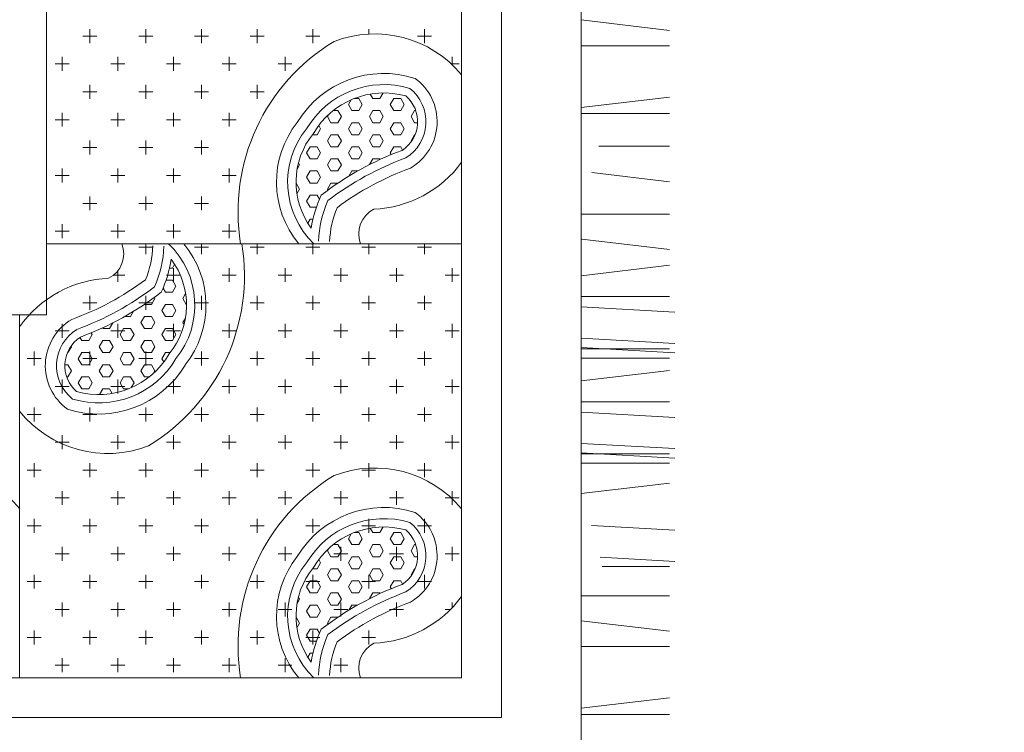
# Model space of a CAD drawing. Units: inches. Extents: x -638 to 186, y -762 to 59.
# Tile 25 of 31: x -65.6 to -46.38, y -107.92 to -94. Entities that reach past the tile are written whole.
import ezdxf

# ---------------------------------------------------------------- set-up
doc = ezdxf.new("R2010")
doc.units = ezdxf.units.IN
doc.layers.add('A-ANNO-DIMS', color=2, linetype='Continuous', lineweight=18)
doc.layers.add('furn', color=8, linetype='Continuous', lineweight=13)
doc.styles.get("Standard").update_dxf_attribs({"font": 'arial.ttf'})
doc.dimstyles.new('ISO-25', dxfattribs={"dimtxt": 4, "dimasz": 4, "dimexe": 1.25, "dimexo": 0.625, "dimtad": 0, "dimlunit": 4, "dimtxsty": 'Standard', "dimcen": 2.5, "dimclrt": 256, "dimadec": 0, "dimazin": 0, "dimtfac": 1, "dimtmove": 0, "dimatfit": 3, "dimfxl": 1, "dimfxlon": 1, "dimarcsym": 0})

# ---------------------------------------------------------------- blocks, each defined once
blk = doc.blocks.new('BED-DOUBLE-WITH-NIGHTSTANDS')
for p, q in [((58.548, 11.244), (58.548, 59.951)), ((68.982, 31.914), (68.982, 1.829)), ((67.427, 30.359), (67.427, 3.384)), ((66.65, 29.582), (66.65, 4.161)), ((68.982, 17.003), (70.71, 16.797)), ((59.394, 16.552), (59.394, 16.825)), ((60.483, 16.552), (60.483, 16.825)), ((61.571, 16.552), (61.571, 16.825)), ((62.659, 16.552), (62.659, 16.825)), ((63.748, 16.552), (63.748, 16.825)), ((64.836, 16.726), (64.836, 16.825)), ((65.924, 16.552), (65.924, 16.825)), ((59.258, 16.688), (59.53, 16.688)), ((60.346, 16.688), (60.619, 16.688)), ((61.435, 16.688), (61.707, 16.688)), ((62.523, 16.688), (62.795, 16.688)), ((63.612, 16.688), (63.884, 16.688)), ((65.788, 16.688), (66.06, 16.688)), ((68.982, 16.497), (70.707, 16.497)), ((58.85, 16.008), (58.85, 16.28)), ((59.938, 16.008), (59.938, 16.28)), ((61.027, 16.008), (61.027, 16.28)), ((62.115, 16.008), (62.115, 16.28)), ((63.203, 16.008), (63.203, 16.28)), ((66.468, 16.127), (66.468, 16.28)), ((58.714, 16.144), (58.986, 16.144)), ((59.802, 16.144), (60.074, 16.144)), ((60.891, 16.144), (61.163, 16.144)), ((61.979, 16.144), (62.251, 16.144)), ((63.067, 16.144), (63.339, 16.144)), ((66.45, 16.144), (66.605, 16.144)), ((59.258, 15.6), (59.53, 15.6)), ((59.394, 15.464), (59.394, 15.736)), ((60.346, 15.6), (60.619, 15.6)), ((60.483, 15.464), (60.483, 15.736)), ((61.435, 15.6), (61.707, 15.6)), ((61.571, 15.464), (61.571, 15.736)), ((62.523, 15.6), (62.795, 15.6)), ((62.659, 15.464), (62.659, 15.736)), ((65.053, 15.469), (65.116, 15.579)), ((64.44, 15.351), (64.495, 15.445)), ((64.552, 15.469), (64.644, 15.469)), ((64.712, 15.351), (64.644, 15.469)), ((64.917, 15.469), (64.866, 15.556)), ((64.917, 15.469), (65.053, 15.469)), ((65.257, 15.351), (65.325, 15.469)), ((65.325, 15.469), (65.461, 15.469)), ((65.529, 15.351), (65.461, 15.469)), ((68.982, 15.294), (70.71, 15.497)), ((58.85, 14.92), (58.85, 15.192)), ((59.938, 14.92), (59.938, 15.192)), ((61.027, 14.92), (61.027, 15.192)), ((62.115, 14.92), (62.115, 15.192)), ((64.143, 15.233), (64.236, 15.233)), ((64.304, 15.115), (64.236, 15.233)), ((64.508, 15.233), (64.44, 15.351)), ((64.508, 15.233), (64.644, 15.233)), ((64.644, 15.233), (64.712, 15.351)), ((64.849, 15.115), (64.917, 15.233)), ((64.917, 15.233), (65.053, 15.233)), ((65.121, 15.115), (65.053, 15.233)), ((65.325, 15.233), (65.257, 15.351)), ((65.325, 15.233), (65.461, 15.233)), ((65.461, 15.233), (65.529, 15.351)), ((65.665, 15.115), (65.733, 15.233)), ((65.733, 15.233), (65.755, 15.233)), ((58.714, 15.056), (58.986, 15.056)), ((59.802, 15.056), (60.074, 15.056)), ((60.891, 15.056), (61.163, 15.056)), ((61.979, 15.056), (62.251, 15.056)), ((64.032, 15.115), (64.059, 15.161)), ((64.1, 14.997), (64.032, 15.115)), ((64.1, 14.997), (64.236, 14.997)), ((64.236, 14.997), (64.304, 15.115)), ((64.44, 14.88), (64.508, 14.997)), ((64.508, 14.997), (64.644, 14.997)), ((64.712, 14.88), (64.644, 14.997)), ((64.917, 14.997), (64.849, 15.115)), ((64.917, 14.997), (65.053, 14.997)), ((65.053, 14.997), (65.121, 15.115)), ((65.257, 14.88), (65.325, 14.997)), ((65.325, 14.997), (65.461, 14.997)), ((65.529, 14.88), (65.461, 14.997)), ((65.733, 14.997), (65.665, 15.115)), ((65.733, 14.997), (65.791, 14.997)), ((68.982, 15.174), (70.707, 15.174)), ((63.828, 14.762), (63.896, 14.88)), ((63.896, 14.88), (63.86, 14.942)), ((64.508, 14.762), (64.44, 14.88)), ((64.644, 14.762), (64.712, 14.88)), ((65.325, 14.762), (65.257, 14.88)), ((65.461, 14.762), (65.529, 14.88)), ((59.394, 14.376), (59.394, 14.648)), ((60.483, 14.376), (60.483, 14.648)), ((61.571, 14.376), (61.571, 14.648)), ((63.737, 14.762), (63.828, 14.762)), ((64.032, 14.644), (64.1, 14.762)), ((64.1, 14.526), (64.032, 14.644)), ((64.1, 14.762), (64.236, 14.762)), ((64.304, 14.644), (64.236, 14.762)), ((64.236, 14.526), (64.304, 14.644)), ((64.508, 14.762), (64.644, 14.762)), ((64.849, 14.644), (64.917, 14.762)), ((64.917, 14.526), (64.849, 14.644)), ((64.917, 14.762), (65.053, 14.762)), ((65.121, 14.644), (65.053, 14.762)), ((65.053, 14.526), (65.121, 14.644)), ((65.325, 14.762), (65.461, 14.762)), ((65.665, 14.644), (65.733, 14.762)), ((65.671, 14.634), (65.665, 14.644)), ((65.733, 14.762), (65.741, 14.762)), ((59.258, 14.512), (59.53, 14.512)), ((60.346, 14.512), (60.619, 14.512)), ((61.435, 14.512), (61.707, 14.512)), ((63.624, 14.408), (63.692, 14.526)), ((63.692, 14.526), (63.828, 14.526)), ((63.896, 14.408), (63.828, 14.526)), ((64.1, 14.526), (64.236, 14.526)), ((64.44, 14.408), (64.508, 14.526)), ((64.508, 14.526), (64.644, 14.526)), ((64.712, 14.408), (64.644, 14.526)), ((64.917, 14.526), (65.053, 14.526)), ((65.257, 14.408), (65.325, 14.526)), ((65.325, 14.526), (65.461, 14.526)), ((65.497, 14.464), (65.461, 14.526)), ((69.331, 14.538), (70.707, 14.538)), ((63.692, 14.291), (63.624, 14.408)), ((63.692, 14.291), (63.828, 14.291)), ((63.828, 14.291), (63.896, 14.408)), ((64.032, 14.173), (64.1, 14.291)), ((64.1, 14.291), (64.236, 14.291)), ((64.304, 14.173), (64.236, 14.291)), ((64.508, 14.291), (64.44, 14.408)), ((64.508, 14.291), (64.644, 14.291)), ((64.644, 14.291), (64.712, 14.408)), ((64.852, 14.179), (64.917, 14.291)), ((64.917, 14.291), (65.053, 14.291)), ((65.059, 14.28), (65.053, 14.291)), ((65.276, 14.375), (65.257, 14.408)), ((58.85, 13.832), (58.85, 14.104)), ((59.938, 13.832), (59.938, 14.104)), ((61.027, 13.832), (61.027, 14.104)), ((62.115, 13.832), (62.115, 14.104)), ((63.438, 14.086), (63.488, 14.173)), ((63.488, 14.173), (63.465, 14.213)), ((63.624, 13.937), (63.692, 14.055)), ((63.692, 14.055), (63.828, 14.055)), ((63.896, 13.937), (63.828, 14.055)), ((64.1, 14.055), (64.032, 14.173)), ((64.1, 14.055), (64.236, 14.055)), ((64.236, 14.055), (64.304, 14.173)), ((64.451, 13.955), (64.508, 14.055)), ((64.508, 14.055), (64.621, 14.055)), ((58.714, 13.968), (58.986, 13.968)), ((59.802, 13.968), (60.074, 13.968)), ((60.891, 13.968), (61.163, 13.968)), ((61.979, 13.968), (62.251, 13.968)), ((63.692, 13.819), (63.624, 13.937)), ((63.828, 13.819), (63.896, 13.937)), ((69.195, 14.023), (70.71, 13.844)), ((63.417, 13.819), (63.42, 13.819)), ((63.488, 13.701), (63.42, 13.819)), ((63.434, 13.608), (63.488, 13.701)), ((63.692, 13.819), (63.828, 13.819)), ((64.032, 13.701), (64.1, 13.819)), ((64.043, 13.682), (64.032, 13.701)), ((64.1, 13.819), (64.236, 13.819)), ((64.237, 13.818), (64.236, 13.819)), ((59.394, 13.287), (59.394, 13.559)), ((60.483, 13.287), (60.483, 13.559)), ((61.571, 13.287), (61.571, 13.559)), ((63.624, 13.466), (63.692, 13.584)), ((63.692, 13.348), (63.624, 13.466)), ((63.692, 13.584), (63.828, 13.584)), ((63.874, 13.504), (63.828, 13.584)), ((59.258, 13.423), (59.53, 13.423)), ((60.346, 13.423), (60.619, 13.423)), ((61.435, 13.423), (61.707, 13.423)), ((63.692, 13.348), (63.815, 13.348)), ((63.648, 13.036), (63.692, 13.112)), ((63.692, 13.112), (63.748, 13.112)), ((68.996, 13.214), (70.707, 13.214)), ((58.85, 12.743), (58.85, 13.015)), ((59.938, 12.743), (59.938, 13.015)), ((61.027, 12.743), (61.027, 13.015)), ((62.115, 12.743), (62.115, 13.015)), ((58.714, 12.879), (58.986, 12.879)), ((59.802, 12.879), (60.074, 12.879)), ((60.891, 12.879), (61.163, 12.879)), ((61.979, 12.879), (62.251, 12.879)), ((68.996, 12.723), (70.71, 12.52)), ((66.65, 12.635), (58.548, 12.635)), ((58.548, 12.635), (66.65, 12.635)), ((60.346, 12.568), (60.619, 12.568)), ((60.483, 12.432), (60.483, 12.635)), ((61.435, 12.568), (61.707, 12.568)), ((61.571, 12.432), (61.571, 12.635)), ((62.523, 12.568), (62.795, 12.568)), ((62.523, 12.568), (62.795, 12.568)), ((62.659, 12.432), (62.659, 12.635)), ((62.659, 12.432), (62.659, 12.635)), ((63.612, 12.568), (63.884, 12.568)), ((63.612, 12.568), (63.884, 12.568)), ((63.748, 12.432), (63.748, 12.635)), ((63.748, 12.432), (63.748, 12.635)), ((64.7, 12.568), (64.972, 12.568)), ((64.7, 12.568), (64.972, 12.568)), ((64.836, 12.432), (64.836, 12.635)), ((64.836, 12.432), (64.836, 12.635)), ((65.788, 12.568), (66.06, 12.568)), ((65.788, 12.568), (66.06, 12.568)), ((65.924, 12.432), (65.924, 12.635)), ((65.924, 12.432), (65.924, 12.635)), ((66.65, 12.635), (66.65, 4.161)), ((61.003, 12.157), (60.948, 12.157)), ((61.047, 12.233), (61.003, 12.157)), ((61.027, 11.888), (61.027, 12.16)), ((62.115, 11.888), (62.115, 12.16)), ((63.203, 11.888), (63.203, 12.16)), ((63.203, 11.888), (63.203, 12.16)), ((64.292, 11.888), (64.292, 12.16)), ((64.292, 11.888), (64.292, 12.16)), ((65.38, 11.888), (65.38, 12.16)), ((65.38, 11.888), (65.38, 12.16)), ((66.468, 11.888), (66.468, 12.16)), ((66.468, 11.888), (66.468, 12.16)), ((68.982, 12.011), (70.71, 12.214)), ((59.857, 12.024), (60.074, 12.024)), ((59.938, 11.888), (59.938, 12.107)), ((61.003, 11.921), (60.881, 11.921)), ((60.891, 12.024), (61.163, 12.024)), ((61.003, 11.921), (61.072, 11.804)), ((61.979, 12.024), (62.251, 12.024)), ((63.067, 12.024), (63.339, 12.024)), ((63.067, 12.024), (63.339, 12.024)), ((64.156, 12.024), (64.428, 12.024)), ((64.156, 12.024), (64.428, 12.024)), ((65.244, 12.024), (65.516, 12.024)), ((65.244, 12.024), (65.516, 12.024)), ((66.332, 12.024), (66.605, 12.024)), ((66.332, 12.024), (66.605, 12.024)), ((60.821, 11.766), (60.867, 11.686)), ((61.072, 11.804), (61.003, 11.686)), ((59.394, 11.344), (59.394, 11.616)), ((60.483, 11.344), (60.483, 11.616)), ((60.663, 11.568), (60.595, 11.45)), ((60.652, 11.587), (60.663, 11.568)), ((61.003, 11.686), (60.867, 11.686)), ((61.261, 11.661), (61.208, 11.568)), ((61.208, 11.568), (61.276, 11.45)), ((61.571, 11.344), (61.571, 11.616)), ((62.659, 11.344), (62.659, 11.616)), ((62.659, 11.344), (62.659, 11.616)), ((63.748, 11.344), (63.748, 11.616)), ((63.748, 11.344), (63.748, 11.616)), ((64.836, 11.344), (64.836, 11.616)), ((64.836, 11.344), (64.836, 11.616)), ((65.924, 11.344), (65.924, 11.616)), ((65.924, 11.344), (65.924, 11.616)), ((68.982, 11.603), (70.71, 11.603)), ((59.258, 11.48), (59.53, 11.48)), ((60.346, 11.48), (60.619, 11.48)), ((60.459, 11.451), (60.459, 11.45)), ((60.595, 11.45), (60.459, 11.45)), ((60.867, 11.45), (60.799, 11.332)), ((61.003, 11.45), (60.867, 11.45)), ((61.003, 11.45), (61.072, 11.332)), ((61.279, 11.45), (61.276, 11.45)), ((61.435, 11.48), (61.707, 11.48)), ((62.523, 11.48), (62.795, 11.48)), ((62.523, 11.48), (62.795, 11.48)), ((63.612, 11.48), (63.884, 11.48)), ((63.612, 11.48), (63.884, 11.48)), ((64.7, 11.48), (64.972, 11.48)), ((64.7, 11.48), (64.972, 11.48)), ((65.788, 11.48), (66.06, 11.48)), ((65.788, 11.48), (66.06, 11.48)), ((68.982, 11.4), (70.811, 11.298)), ((20.158, 11.244), (58.548, 11.244)), ((58.022, 4.161), (58.022, 11.244)), ((58.022, 11.244), (58.022, 4.161)), ((60.187, 11.215), (60.075, 11.215)), ((60.245, 11.315), (60.187, 11.215)), ((60.459, 11.215), (60.391, 11.097)), ((60.595, 11.215), (60.459, 11.215)), ((60.595, 11.215), (60.663, 11.097)), ((60.799, 11.332), (60.867, 11.215)), ((61.003, 11.215), (60.867, 11.215)), ((61.072, 11.332), (61.003, 11.215)), ((61.258, 11.184), (61.208, 11.097)), ((58.85, 10.8), (58.85, 11.072)), ((59.637, 10.99), (59.643, 10.979)), ((59.779, 10.979), (59.643, 10.979)), ((59.843, 11.09), (59.779, 10.979)), ((59.938, 10.8), (59.938, 11.072)), ((60.051, 10.979), (59.983, 10.861)), ((60.187, 10.979), (60.051, 10.979)), ((60.187, 10.979), (60.255, 10.861)), ((60.391, 11.097), (60.459, 10.979)), ((60.595, 10.979), (60.459, 10.979)), ((60.663, 11.097), (60.595, 10.979)), ((60.867, 10.979), (60.799, 10.861)), ((61.003, 10.979), (60.867, 10.979)), ((61.003, 10.979), (61.072, 10.861)), ((61.027, 10.8), (61.027, 11.072)), ((61.208, 11.097), (61.231, 11.057)), ((62.115, 10.8), (62.115, 11.072)), ((63.203, 10.8), (63.203, 11.072)), ((63.203, 10.8), (63.203, 11.072)), ((64.292, 10.8), (64.292, 11.072)), ((64.292, 10.8), (64.292, 11.072)), ((65.38, 10.8), (65.38, 11.072)), ((65.38, 10.8), (65.38, 11.072)), ((66.468, 10.8), (66.468, 11.072)), ((66.468, 10.8), (66.468, 11.072)), ((58.714, 10.936), (58.986, 10.936)), ((59.199, 10.806), (59.235, 10.743)), ((59.439, 10.861), (59.371, 10.743)), ((59.419, 10.895), (59.439, 10.861)), ((59.802, 10.936), (60.074, 10.936)), ((59.983, 10.861), (60.051, 10.743)), ((60.255, 10.861), (60.187, 10.743)), ((60.799, 10.861), (60.867, 10.743)), ((60.891, 10.936), (61.163, 10.936)), ((61.072, 10.861), (61.003, 10.743)), ((61.979, 10.936), (62.251, 10.936)), ((63.067, 10.936), (63.339, 10.936)), ((63.067, 10.936), (63.339, 10.936)), ((64.156, 10.936), (64.428, 10.936)), ((64.156, 10.936), (64.428, 10.936)), ((65.244, 10.936), (65.516, 10.936)), ((65.244, 10.936), (65.516, 10.936)), ((66.332, 10.936), (66.605, 10.936)), ((66.332, 10.936), (66.605, 10.936)), ((68.982, 10.789), (70.811, 10.687)), ((59.031, 10.625), (58.963, 10.508)), ((59.025, 10.636), (59.031, 10.625)), ((59.371, 10.743), (59.235, 10.743)), ((59.643, 10.743), (59.575, 10.625)), ((59.575, 10.625), (59.643, 10.508)), ((59.779, 10.743), (59.643, 10.743)), ((59.779, 10.743), (59.847, 10.625)), ((59.847, 10.625), (59.779, 10.508)), ((60.187, 10.743), (60.051, 10.743)), ((60.459, 10.743), (60.391, 10.625)), ((60.391, 10.625), (60.459, 10.508)), ((60.595, 10.743), (60.459, 10.743)), ((60.595, 10.743), (60.663, 10.625)), ((60.663, 10.625), (60.595, 10.508)), ((61.003, 10.743), (60.867, 10.743)), ((68.982, 10.606), (70.811, 10.504)), ((68.982, 10.585), (70.71, 10.585)), ((58.17, 10.392), (58.442, 10.392)), ((58.306, 10.256), (58.306, 10.528)), ((58.963, 10.508), (58.955, 10.508)), ((59.235, 10.508), (59.167, 10.39)), ((59.167, 10.39), (59.235, 10.272)), ((59.371, 10.508), (59.235, 10.508)), ((59.258, 10.392), (59.53, 10.392)), ((59.371, 10.508), (59.439, 10.39)), ((59.439, 10.39), (59.371, 10.272)), ((59.394, 10.256), (59.394, 10.528)), ((59.779, 10.508), (59.643, 10.508)), ((60.051, 10.508), (59.983, 10.39)), ((59.983, 10.39), (60.051, 10.272)), ((60.187, 10.508), (60.051, 10.508)), ((60.187, 10.508), (60.255, 10.39)), ((60.255, 10.39), (60.187, 10.272)), ((60.346, 10.392), (60.619, 10.392)), ((60.595, 10.508), (60.459, 10.508)), ((60.483, 10.256), (60.483, 10.528)), ((60.867, 10.508), (60.799, 10.39)), ((60.799, 10.39), (60.836, 10.327)), ((60.958, 10.508), (60.867, 10.508)), ((61.435, 10.392), (61.707, 10.392)), ((61.571, 10.256), (61.571, 10.528)), ((62.523, 10.392), (62.795, 10.392)), ((62.523, 10.392), (62.795, 10.392)), ((62.659, 10.256), (62.659, 10.528)), ((62.659, 10.256), (62.659, 10.528)), ((63.612, 10.392), (63.884, 10.392)), ((63.612, 10.392), (63.884, 10.392)), ((63.748, 10.256), (63.748, 10.528)), ((63.748, 10.256), (63.748, 10.528)), ((64.7, 10.392), (64.972, 10.392)), ((64.7, 10.392), (64.972, 10.392)), ((64.836, 10.256), (64.836, 10.528)), ((64.836, 10.256), (64.836, 10.528)), ((65.788, 10.392), (66.06, 10.392)), ((65.788, 10.392), (66.06, 10.392)), ((65.924, 10.256), (65.924, 10.528)), ((65.924, 10.256), (65.924, 10.528)), ((68.982, 10.402), (70.71, 10.402)), ((58.963, 10.272), (58.904, 10.272)), ((58.963, 10.272), (59.031, 10.154)), ((59.371, 10.272), (59.235, 10.272)), ((59.643, 10.272), (59.575, 10.154)), ((59.779, 10.272), (59.643, 10.272)), ((59.779, 10.272), (59.847, 10.154)), ((60.187, 10.272), (60.051, 10.272)), ((60.459, 10.272), (60.391, 10.154)), ((60.595, 10.272), (60.459, 10.272)), ((60.595, 10.272), (60.663, 10.154)), ((58.963, 10.036), (58.94, 10.036)), ((59.031, 10.154), (58.963, 10.036)), ((59.235, 10.036), (59.167, 9.919)), ((59.371, 10.036), (59.235, 10.036)), ((59.371, 10.036), (59.439, 9.919)), ((59.575, 10.154), (59.643, 10.036)), ((59.779, 10.036), (59.643, 10.036)), ((59.847, 10.154), (59.779, 10.036)), ((60.051, 10.036), (59.983, 9.919)), ((60.187, 10.036), (60.051, 10.036)), ((60.187, 10.036), (60.255, 9.919)), ((60.391, 10.154), (60.459, 10.036)), ((60.553, 10.036), (60.459, 10.036)), ((60.663, 10.154), (60.637, 10.108)), ((68.982, 9.957), (70.71, 10.161)), ((58.714, 9.847), (58.986, 9.847)), ((58.85, 9.711), (58.85, 9.983)), ((59.167, 9.919), (59.235, 9.801)), ((59.439, 9.919), (59.371, 9.801)), ((59.802, 9.847), (60.074, 9.847)), ((59.938, 9.711), (59.938, 9.983)), ((59.983, 9.919), (60.051, 9.801)), ((60.255, 9.919), (60.201, 9.825)), ((60.891, 9.847), (61.163, 9.847)), ((61.027, 9.711), (61.027, 9.983)), ((61.979, 9.847), (62.251, 9.847)), ((61.979, 9.847), (62.251, 9.847)), ((62.115, 9.711), (62.115, 9.983)), ((62.115, 9.711), (62.115, 9.983)), ((63.067, 9.847), (63.339, 9.847)), ((63.067, 9.847), (63.339, 9.847)), ((63.203, 9.711), (63.203, 9.983)), ((63.203, 9.711), (63.203, 9.983)), ((64.156, 9.847), (64.428, 9.847)), ((64.156, 9.847), (64.428, 9.847)), ((64.292, 9.711), (64.292, 9.983)), ((64.292, 9.711), (64.292, 9.983)), ((65.244, 9.847), (65.516, 9.847)), ((65.244, 9.847), (65.516, 9.847)), ((65.38, 9.711), (65.38, 9.983)), ((65.38, 9.711), (65.38, 9.983)), ((66.332, 9.847), (66.605, 9.847)), ((66.332, 9.847), (66.605, 9.847)), ((66.468, 9.711), (66.468, 9.983)), ((66.468, 9.711), (66.468, 9.983)), ((59.371, 9.801), (59.235, 9.801)), ((59.643, 9.801), (59.58, 9.691)), ((59.779, 9.801), (59.643, 9.801)), ((59.779, 9.801), (59.83, 9.713)), ((60.144, 9.801), (60.051, 9.801)), ((58.306, 9.167), (58.306, 9.439)), ((59.394, 9.167), (59.394, 9.439)), ((60.483, 9.167), (60.483, 9.439)), ((61.571, 9.167), (61.571, 9.439)), ((61.571, 9.167), (61.571, 9.439)), ((62.659, 9.167), (62.659, 9.439)), ((62.659, 9.167), (62.659, 9.439)), ((63.748, 9.167), (63.748, 9.439)), ((63.748, 9.167), (63.748, 9.439)), ((64.836, 9.167), (64.836, 9.439)), ((64.836, 9.167), (64.836, 9.439)), ((65.924, 9.167), (65.924, 9.439)), ((65.924, 9.167), (65.924, 9.439)), ((68.982, 9.55), (70.71, 9.55)), ((58.17, 9.303), (58.442, 9.303)), ((59.258, 9.303), (59.53, 9.303)), ((60.346, 9.303), (60.619, 9.303)), ((61.435, 9.303), (61.707, 9.303)), ((61.435, 9.303), (61.707, 9.303)), ((62.523, 9.303), (62.795, 9.303)), ((62.523, 9.303), (62.795, 9.303)), ((63.612, 9.303), (63.884, 9.303)), ((63.612, 9.303), (63.884, 9.303)), ((64.7, 9.303), (64.972, 9.303)), ((64.7, 9.303), (64.972, 9.303)), ((65.788, 9.303), (66.06, 9.303)), ((65.788, 9.303), (66.06, 9.303)), ((68.982, 9.347), (70.811, 9.245)), ((58.85, 8.623), (58.85, 8.895)), ((59.938, 8.623), (59.938, 8.895)), ((61.027, 8.623), (61.027, 8.895)), ((61.027, 8.623), (61.027, 8.895)), ((62.115, 8.623), (62.115, 8.895)), ((62.115, 8.623), (62.115, 8.895)), ((63.203, 8.623), (63.203, 8.895)), ((63.203, 8.623), (63.203, 8.895)), ((64.292, 8.623), (64.292, 8.895)), ((64.292, 8.623), (64.292, 8.895)), ((65.38, 8.623), (65.38, 8.895)), ((65.38, 8.623), (65.38, 8.895)), ((66.468, 8.623), (66.468, 8.895)), ((66.468, 8.623), (66.468, 8.895)), ((58.714, 8.759), (58.783, 8.759)), ((58.714, 8.759), (58.986, 8.759)), ((58.85, 8.623), (58.85, 8.728)), ((59.802, 8.759), (60.074, 8.759)), ((60.891, 8.759), (61.163, 8.759)), ((60.891, 8.759), (61.163, 8.759)), ((61.979, 8.759), (62.251, 8.759)), ((61.979, 8.759), (62.251, 8.759)), ((63.067, 8.759), (63.339, 8.759)), ((63.067, 8.759), (63.339, 8.759)), ((64.156, 8.759), (64.428, 8.759)), ((64.156, 8.759), (64.428, 8.759)), ((65.244, 8.759), (65.516, 8.759)), ((65.244, 8.759), (65.516, 8.759)), ((66.332, 8.759), (66.605, 8.759)), ((66.332, 8.759), (66.605, 8.759)), ((68.982, 8.736), (70.811, 8.634)), ((68.982, 8.553), (70.811, 8.451)), ((68.982, 8.532), (70.71, 8.532)), ((58.306, 8.079), (58.306, 8.351)), ((58.306, 8.079), (58.306, 8.351)), ((59.394, 8.079), (59.394, 8.351)), ((59.394, 8.079), (59.394, 8.351)), ((60.483, 8.079), (60.483, 8.351)), ((60.483, 8.079), (60.483, 8.351)), ((61.571, 8.079), (61.571, 8.351)), ((61.571, 8.079), (61.571, 8.351)), ((62.659, 8.079), (62.659, 8.351)), ((62.659, 8.079), (62.659, 8.351)), ((63.748, 8.079), (63.748, 8.351)), ((63.748, 8.079), (63.748, 8.351)), ((64.836, 8.253), (64.836, 8.351)), ((64.836, 8.079), (64.836, 8.351)), ((65.924, 8.079), (65.924, 8.351)), ((65.924, 8.079), (65.924, 8.351)), ((68.982, 8.349), (70.71, 8.349)), ((58.17, 8.215), (58.442, 8.215)), ((58.17, 8.215), (58.442, 8.215)), ((59.258, 8.215), (59.53, 8.215)), ((59.258, 8.215), (59.53, 8.215)), ((60.346, 8.215), (60.619, 8.215)), ((60.346, 8.215), (60.619, 8.215)), ((61.435, 8.215), (61.707, 8.215)), ((61.435, 8.215), (61.707, 8.215)), ((62.523, 8.215), (62.795, 8.215)), ((62.523, 8.215), (62.795, 8.215)), ((63.612, 8.215), (63.884, 8.215)), ((63.612, 8.215), (63.884, 8.215)), ((64.7, 8.215), (64.972, 8.215)), ((65.788, 8.215), (66.06, 8.215)), ((65.788, 8.215), (66.06, 8.215)), ((68.982, 7.757), (70.71, 7.961)), ((58.85, 7.535), (58.85, 7.807)), ((58.85, 7.535), (58.85, 7.807)), ((59.938, 7.535), (59.938, 7.807)), ((59.938, 7.535), (59.938, 7.807)), ((61.027, 7.535), (61.027, 7.807)), ((61.027, 7.535), (61.027, 7.807)), ((62.115, 7.535), (62.115, 7.807)), ((62.115, 7.535), (62.115, 7.807)), ((63.203, 7.535), (63.203, 7.807)), ((63.203, 7.535), (63.203, 7.807)), ((64.292, 7.535), (64.292, 7.807)), ((65.38, 7.535), (65.38, 7.807)), ((66.468, 7.653), (66.468, 7.807)), ((66.468, 7.535), (66.468, 7.807)), ((58.714, 7.671), (58.986, 7.671)), ((58.714, 7.671), (58.986, 7.671)), ((59.802, 7.671), (60.074, 7.671)), ((59.802, 7.671), (60.074, 7.671)), ((60.891, 7.671), (61.163, 7.671)), ((60.891, 7.671), (61.163, 7.671)), ((61.979, 7.671), (62.251, 7.671)), ((61.979, 7.671), (62.251, 7.671)), ((63.067, 7.671), (63.339, 7.671)), ((63.067, 7.671), (63.339, 7.671)), ((64.156, 7.671), (64.428, 7.671)), ((65.244, 7.671), (65.516, 7.671)), ((66.332, 7.671), (66.605, 7.671)), ((66.45, 7.671), (66.605, 7.671)), ((58.17, 7.127), (58.442, 7.127)), ((58.17, 7.127), (58.442, 7.127)), ((58.306, 6.99), (58.306, 7.263)), ((58.306, 6.99), (58.306, 7.263)), ((59.258, 7.127), (59.53, 7.127)), ((59.258, 7.127), (59.53, 7.127)), ((59.394, 6.99), (59.394, 7.263)), ((59.394, 6.99), (59.394, 7.263)), ((60.346, 7.127), (60.619, 7.127)), ((60.346, 7.127), (60.619, 7.127)), ((60.483, 6.99), (60.483, 7.263)), ((60.483, 6.99), (60.483, 7.263)), ((61.435, 7.127), (61.707, 7.127)), ((61.435, 7.127), (61.707, 7.127)), ((61.571, 6.99), (61.571, 7.263)), ((61.571, 6.99), (61.571, 7.263)), ((62.523, 7.127), (62.795, 7.127)), ((62.523, 7.127), (62.795, 7.127)), ((62.659, 6.99), (62.659, 7.263)), ((62.659, 6.99), (62.659, 7.263)), ((63.612, 7.127), (63.884, 7.127)), ((63.748, 6.99), (63.748, 7.263)), ((64.7, 7.127), (64.972, 7.127)), ((64.836, 6.99), (64.836, 7.263)), ((65.788, 7.127), (66.06, 7.127)), ((65.924, 6.99), (65.924, 7.263)), ((69.184, 7.135), (70.811, 7.044)), ((64.44, 6.877), (64.495, 6.971)), ((64.552, 6.995), (64.644, 6.995)), ((64.712, 6.877), (64.644, 6.995)), ((64.917, 6.995), (64.866, 7.082)), ((64.917, 6.995), (65.053, 6.995)), ((65.053, 6.995), (65.116, 7.105)), ((65.257, 6.877), (65.325, 6.995)), ((65.325, 6.995), (65.461, 6.995)), ((65.529, 6.877), (65.461, 6.995)), ((64.143, 6.76), (64.236, 6.76)), ((64.304, 6.642), (64.236, 6.76)), ((64.508, 6.76), (64.44, 6.877)), ((64.508, 6.76), (64.644, 6.76)), ((64.644, 6.76), (64.712, 6.877)), ((64.849, 6.642), (64.917, 6.76)), ((64.917, 6.76), (65.053, 6.76)), ((65.121, 6.642), (65.053, 6.76)), ((65.325, 6.76), (65.257, 6.877)), ((65.325, 6.76), (65.461, 6.76)), ((65.461, 6.76), (65.529, 6.877)), ((65.665, 6.642), (65.733, 6.76)), ((65.733, 6.76), (65.755, 6.76)), ((58.714, 6.582), (58.986, 6.582)), ((58.714, 6.582), (58.986, 6.582)), ((58.85, 6.446), (58.85, 6.718)), ((58.85, 6.446), (58.85, 6.718)), ((59.802, 6.582), (60.074, 6.582)), ((59.802, 6.582), (60.074, 6.582)), ((59.938, 6.446), (59.938, 6.718)), ((59.938, 6.446), (59.938, 6.718)), ((60.891, 6.582), (61.163, 6.582)), ((60.891, 6.582), (61.163, 6.582)), ((61.027, 6.446), (61.027, 6.718)), ((61.027, 6.446), (61.027, 6.718)), ((61.979, 6.582), (62.251, 6.582)), ((61.979, 6.582), (62.251, 6.582)), ((62.115, 6.446), (62.115, 6.718)), ((62.115, 6.446), (62.115, 6.718)), ((63.067, 6.582), (63.339, 6.582)), ((63.203, 6.446), (63.203, 6.718)), ((64.032, 6.642), (64.059, 6.688)), ((64.1, 6.524), (64.032, 6.642)), ((64.156, 6.582), (64.428, 6.582)), ((64.236, 6.524), (64.304, 6.642)), ((64.292, 6.446), (64.292, 6.718)), ((64.917, 6.524), (64.849, 6.642)), ((65.053, 6.524), (65.121, 6.642)), ((65.244, 6.582), (65.516, 6.582)), ((65.38, 6.446), (65.38, 6.718)), ((65.733, 6.524), (65.665, 6.642)), ((66.332, 6.582), (66.605, 6.582)), ((66.468, 6.446), (66.468, 6.718)), ((63.828, 6.288), (63.896, 6.406)), ((63.896, 6.406), (63.86, 6.469)), ((64.1, 6.524), (64.236, 6.524)), ((64.44, 6.406), (64.508, 6.524)), ((64.508, 6.288), (64.44, 6.406)), ((64.508, 6.524), (64.644, 6.524)), ((64.712, 6.406), (64.644, 6.524)), ((64.644, 6.288), (64.712, 6.406)), ((64.917, 6.524), (65.053, 6.524)), ((65.257, 6.406), (65.325, 6.524)), ((65.325, 6.288), (65.257, 6.406)), ((65.325, 6.524), (65.461, 6.524)), ((65.529, 6.406), (65.461, 6.524)), ((65.461, 6.288), (65.529, 6.406)), ((65.733, 6.524), (65.791, 6.524)), ((69.357, 6.514), (70.811, 6.433)), ((58.306, 5.902), (58.306, 6.174)), ((58.306, 5.902), (58.306, 6.174)), ((59.394, 5.902), (59.394, 6.174)), ((59.394, 5.902), (59.394, 6.174)), ((60.483, 5.902), (60.483, 6.174)), ((60.483, 5.902), (60.483, 6.174)), ((61.571, 5.902), (61.571, 6.174)), ((61.571, 5.902), (61.571, 6.174)), ((62.659, 5.902), (62.659, 6.174)), ((63.737, 6.288), (63.828, 6.288)), ((63.748, 5.902), (63.748, 6.174)), ((64.032, 6.17), (64.1, 6.288)), ((64.1, 6.053), (64.032, 6.17)), ((64.1, 6.288), (64.236, 6.288)), ((64.304, 6.17), (64.236, 6.288)), ((64.236, 6.053), (64.304, 6.17)), ((64.508, 6.288), (64.644, 6.288)), ((64.836, 5.902), (64.836, 6.174)), ((64.849, 6.17), (64.917, 6.288)), ((64.917, 6.053), (64.849, 6.17)), ((64.917, 6.288), (65.053, 6.288)), ((65.121, 6.17), (65.053, 6.288)), ((65.053, 6.053), (65.121, 6.17)), ((65.325, 6.288), (65.461, 6.288)), ((65.665, 6.17), (65.733, 6.288)), ((65.671, 6.16), (65.665, 6.17)), ((65.733, 6.288), (65.741, 6.288)), ((65.924, 5.902), (65.924, 6.174)), ((69.393, 6.332), (70.71, 6.332)), ((58.17, 6.038), (58.442, 6.038)), ((58.17, 6.038), (58.442, 6.038)), ((59.258, 6.038), (59.53, 6.038)), ((59.258, 6.038), (59.53, 6.038)), ((60.346, 6.038), (60.619, 6.038)), ((60.346, 6.038), (60.619, 6.038)), ((61.435, 6.038), (61.707, 6.038)), ((61.435, 6.038), (61.707, 6.038)), ((62.523, 6.038), (62.795, 6.038)), ((63.612, 6.038), (63.884, 6.038)), ((63.624, 5.935), (63.692, 6.053)), ((63.692, 6.053), (63.828, 6.053)), ((63.896, 5.935), (63.828, 6.053)), ((64.1, 6.053), (64.236, 6.053)), ((64.44, 5.935), (64.508, 6.053)), ((64.508, 6.053), (64.644, 6.053)), ((64.712, 5.935), (64.644, 6.053)), ((64.7, 6.038), (64.972, 6.038)), ((64.917, 6.053), (65.053, 6.053)), ((65.257, 5.935), (65.325, 6.053)), ((65.325, 6.053), (65.461, 6.053)), ((65.497, 5.99), (65.461, 6.053)), ((65.788, 6.038), (66.06, 6.038)), ((63.692, 5.817), (63.624, 5.935)), ((63.692, 5.817), (63.828, 5.817)), ((63.828, 5.817), (63.896, 5.935)), ((64.032, 5.699), (64.1, 5.817)), ((64.1, 5.817), (64.236, 5.817)), ((64.304, 5.699), (64.236, 5.817)), ((64.508, 5.817), (64.44, 5.935)), ((64.508, 5.817), (64.644, 5.817)), ((64.644, 5.817), (64.712, 5.935)), ((64.852, 5.706), (64.917, 5.817)), ((64.917, 5.817), (65.053, 5.817)), ((65.059, 5.806), (65.053, 5.817)), ((65.276, 5.901), (65.257, 5.935)), ((58.85, 5.358), (58.85, 5.63)), ((58.85, 5.358), (58.85, 5.63)), ((59.938, 5.358), (59.938, 5.63)), ((59.938, 5.358), (59.938, 5.63)), ((61.027, 5.358), (61.027, 5.63)), ((61.027, 5.358), (61.027, 5.63)), ((62.115, 5.358), (62.115, 5.63)), ((62.115, 5.358), (62.115, 5.63)), ((63.203, 5.358), (63.203, 5.63)), ((63.438, 5.612), (63.488, 5.699)), ((63.488, 5.699), (63.465, 5.739)), ((63.624, 5.464), (63.692, 5.581)), ((63.692, 5.581), (63.828, 5.581)), ((63.896, 5.464), (63.828, 5.581)), ((64.1, 5.581), (64.032, 5.699)), ((64.1, 5.581), (64.236, 5.581)), ((64.236, 5.581), (64.304, 5.699)), ((64.292, 5.358), (64.292, 5.63)), ((64.451, 5.481), (64.508, 5.581)), ((64.508, 5.581), (64.621, 5.581)), ((65.38, 5.358), (65.38, 5.63)), ((66.468, 5.533), (66.468, 5.63)), ((68.982, 5.764), (70.707, 5.764)), ((58.714, 5.494), (58.986, 5.494)), ((58.714, 5.494), (58.986, 5.494)), ((59.802, 5.494), (60.074, 5.494)), ((59.802, 5.494), (60.074, 5.494)), ((60.891, 5.494), (61.163, 5.494)), ((60.891, 5.494), (61.163, 5.494)), ((61.979, 5.494), (62.251, 5.494)), ((61.979, 5.494), (62.251, 5.494)), ((63.067, 5.494), (63.339, 5.494)), ((63.692, 5.346), (63.624, 5.464)), ((63.828, 5.346), (63.896, 5.464)), ((64.156, 5.494), (64.428, 5.494)), ((65.244, 5.494), (65.516, 5.494)), ((66.332, 5.494), (66.43, 5.494)), ((63.417, 5.346), (63.42, 5.346)), ((63.488, 5.228), (63.42, 5.346)), ((63.434, 5.135), (63.488, 5.228)), ((63.692, 5.346), (63.828, 5.346)), ((64.032, 5.228), (64.1, 5.346)), ((64.043, 5.209), (64.032, 5.228)), ((64.1, 5.346), (64.236, 5.346)), ((64.237, 5.344), (64.236, 5.346)), ((68.982, 5.274), (70.71, 5.069)), ((58.306, 4.814), (58.306, 5.086)), ((58.306, 4.814), (58.306, 5.086)), ((59.394, 4.814), (59.394, 5.086)), ((59.394, 4.814), (59.394, 5.086)), ((60.483, 4.814), (60.483, 5.086)), ((60.483, 4.814), (60.483, 5.086)), ((61.571, 4.814), (61.571, 5.086)), ((61.571, 4.814), (61.571, 5.086)), ((62.659, 4.814), (62.659, 5.086)), ((63.624, 4.992), (63.692, 5.11)), ((63.692, 5.11), (63.828, 5.11)), ((63.748, 4.814), (63.748, 5.086)), ((63.874, 5.03), (63.828, 5.11)), ((64.836, 4.814), (64.836, 5.086)), ((58.17, 4.95), (58.442, 4.95)), ((58.17, 4.95), (58.442, 4.95)), ((59.258, 4.95), (59.53, 4.95)), ((59.258, 4.95), (59.53, 4.95)), ((60.346, 4.95), (60.619, 4.95)), ((60.346, 4.95), (60.619, 4.95)), ((61.435, 4.95), (61.707, 4.95)), ((61.435, 4.95), (61.707, 4.95)), ((62.523, 4.95), (62.795, 4.95)), ((63.612, 4.95), (63.884, 4.95)), ((63.692, 4.874), (63.624, 4.992)), ((63.692, 4.874), (63.815, 4.874)), ((64.7, 4.95), (64.972, 4.95)), ((63.648, 4.563), (63.692, 4.639)), ((63.692, 4.639), (63.748, 4.639)), ((68.982, 4.769), (70.707, 4.769)), ((58.85, 4.27), (58.85, 4.542)), ((58.85, 4.27), (58.85, 4.542)), ((59.938, 4.27), (59.938, 4.542)), ((59.938, 4.27), (59.938, 4.542)), ((61.027, 4.27), (61.027, 4.542)), ((61.027, 4.27), (61.027, 4.542)), ((62.115, 4.27), (62.115, 4.542)), ((62.115, 4.27), (62.115, 4.542)), ((63.203, 4.27), (63.203, 4.542)), ((64.292, 4.27), (64.292, 4.542)), ((58.714, 4.406), (58.986, 4.406)), ((58.714, 4.406), (58.986, 4.406)), ((59.802, 4.406), (60.074, 4.406)), ((59.802, 4.406), (60.074, 4.406)), ((60.891, 4.406), (61.163, 4.406)), ((60.891, 4.406), (61.163, 4.406)), ((61.979, 4.406), (62.251, 4.406)), ((61.979, 4.406), (62.251, 4.406)), ((63.067, 4.406), (63.339, 4.406)), ((64.156, 4.406), (64.428, 4.406)), ((66.65, 4.161), (40.767, 4.161)), ((66.65, 4.161), (58.022, 4.161)), ((68.982, 3.565), (70.71, 3.769)), ((67.427, 3.384), (39.99, 3.384)), ((68.982, 3.446), (70.707, 3.446))]:
    blk.add_line(p, q)
for centre, radius, start, end in [((64.955, 14.528), 2.202, 39.6653, 111.1583), ((66.165, 13.26), 3.88, 121.1125, 189.2666), ((65.133, 13.987), 1.972, 72.055, 149.019), ((65.126, 15.016), 1.047, 300.344, 54.0192), ((65.133, 13.987), 1.754, 73.2189, 149.4808), ((65.133, 13.987), 1.591, 74.3738, 149.9117), ((65.126, 15.016), 0.829, 301.6232, 51.6957), ((65.126, 15.016), 0.666, 302.9498, 49.099), ((64.914, 13.836), 1.878, 141.5973, 219.7611), ((64.914, 13.836), 1.66, 141.1107, 226.3387), ((64.914, 13.836), 1.497, 140.6541, 216.833), ((67.553, 8.875), 5.952, 110.2997, 127.7385), ((67.553, 8.875), 5.789, 110.1318, 127.346), ((67.553, 8.875), 5.571, 109.9219, 126.7677), ((64.84, 15.553), 2.246, 272.4675, 323.7193), ((65.96, 12.613), 2.268, 154.7059, 171.7535), ((65.96, 12.613), 2.104, 155.7609, 178.0373), ((65.96, 12.613), 1.887, 157.4091, 178.0373), ((65.181, 12.828), 0.54, 117.0088, 201.0409), ((59.514, 12.441), 0.54, 297.0088, 21.0409), ((58.736, 12.656), 1.887, 337.4091, 358.0373), ((58.53, 12.01), 3.88, 301.1125, 9.2666), ((58.736, 12.656), 2.104, 335.7609, 358.0373), ((59.782, 11.434), 1.66, 321.1107, 46.3387), ((59.782, 11.434), 1.878, 321.5973, 39.7611), ((58.736, 12.656), 2.268, 334.7059, 351.7535), ((59.782, 11.434), 1.497, 320.6541, 36.833), ((59.856, 9.717), 2.246, 92.4675, 144.7393), ((57.143, 16.395), 5.571, 289.9219, 306.7677), ((57.143, 16.395), 5.789, 290.1318, 307.346), ((57.143, 16.395), 5.952, 290.2997, 307.7385), ((59.57, 10.253), 1.047, 120.344, 234.0192), ((59.57, 10.253), 0.829, 121.6232, 231.6957), ((59.57, 10.253), 0.666, 122.9498, 229.099), ((59.563, 11.282), 1.754, 253.2189, 329.4808), ((59.563, 11.282), 1.591, 254.3738, 329.9117), ((59.563, 11.282), 1.972, 252.055, 329.019), ((59.74, 10.742), 2.202, 218.7027, 291.1583), ((56.328, 6.054), 2.202, 39.6653, 111.1583), ((66.165, 4.786), 3.88, 121.1125, 189.2666), ((64.955, 6.054), 2.202, 39.6653, 111.1583), ((65.133, 5.514), 1.972, 72.055, 149.019), ((65.126, 6.543), 1.047, 300.344, 54.0192), ((65.133, 5.514), 1.754, 73.2189, 149.4808), ((65.126, 6.543), 0.829, 301.6232, 51.6957), ((65.133, 5.514), 1.591, 74.3738, 149.9117), ((65.126, 6.543), 0.666, 302.9498, 49.099), ((64.914, 5.362), 1.878, 141.5973, 219.7611), ((64.914, 5.362), 1.66, 141.1107, 226.3387), ((64.914, 5.362), 1.497, 140.6541, 216.833), ((67.553, 0.401), 5.952, 110.2997, 127.7385), ((67.553, 0.401), 5.789, 110.1318, 127.346), ((67.553, 0.401), 5.571, 109.9219, 126.7677), ((64.84, 7.079), 2.246, 272.4675, 323.7193), ((65.96, 4.14), 2.268, 154.7059, 171.7535), ((65.96, 4.14), 2.104, 155.7609, 178.0373), ((65.96, 4.14), 1.887, 157.4091, 178.0373), ((65.181, 4.355), 0.54, 117.0088, 201.0409)]:
    blk.add_arc(centre, radius, start, end)
blk = doc.blocks.new('*D27')
at = {"layer": 'A-ANNO-DIMS', "color": 0, "lineweight": -2, "transparency": 16777216}
for p, q in [((-123.625, -121.818), (-123.625, -124.068)), ((-44.925, -121.818), (-44.925, -124.068)), ((-119.625, -122.818), (-114.394, -122.818)), ((-48.925, -122.818), (-54.156, -122.818))]:
    blk.add_line(p, q, dxfattribs=at)
at = {"layer": 'A-ANNO-DIMS', "color": 0, "lineweight": 30, "transparency": 16777216}
for points in [[(-119.625, -122.151), (-119.625, -123.485), (-123.625, -122.818)], [(-48.925, -122.151), (-48.925, -123.485), (-44.925, -122.818)]]:
    blk.add_solid(points, dxfattribs=at)
at = {"layer": 'Defpoints', "color": 0, "lineweight": 30, "transparency": 16777216}
for p in [(-123.625, -111.013), (-44.925, -111.013), (-44.925, -122.818)]:
    blk.add_point(p, dxfattribs=at)
at = {"layer": 'A-ANNO-DIMS', "transparency": 16777216, "insert": (-84.275, -122.818), "char_height": 4, "attachment_point": 5}
blk.add_mtext('BED SET 6\'-6 1/2" TYP.', dxfattribs=at)

msp = doc.modelspace()

# ---------------------------------------------------------------- block references
at = {"layer": 'furn'}
msp.add_blockref('BED-DOUBLE-WITH-NIGHTSTANDS', (-123.625, -111.013), dxfattribs=at)

# ---------------------------------------------------------------- dimensions: what is measured, and where the dimension line sits
at = {"layer": 'A-ANNO-DIMS'}
dim = msp.add_linear_dim(base=(-44.925, -122.818), p1=(-123.625, -111.013), p2=(-44.925, -111.013), text='BED SET <> TYP.', dimstyle='ISO-25', override={"dimdec": 1, "dimlfac": 1, "dimrnd": 0, "dimzin": 1, "dimdsep": 46, "dimlunit": 4, "dimfrac": 2}, dxfattribs=at)
dim.commit()
dim.dimension.update_dxf_attribs({"geometry": '*D27', "text_midpoint": (-84.275, -122.818)})

doc.saveas('drawing.dxf')
